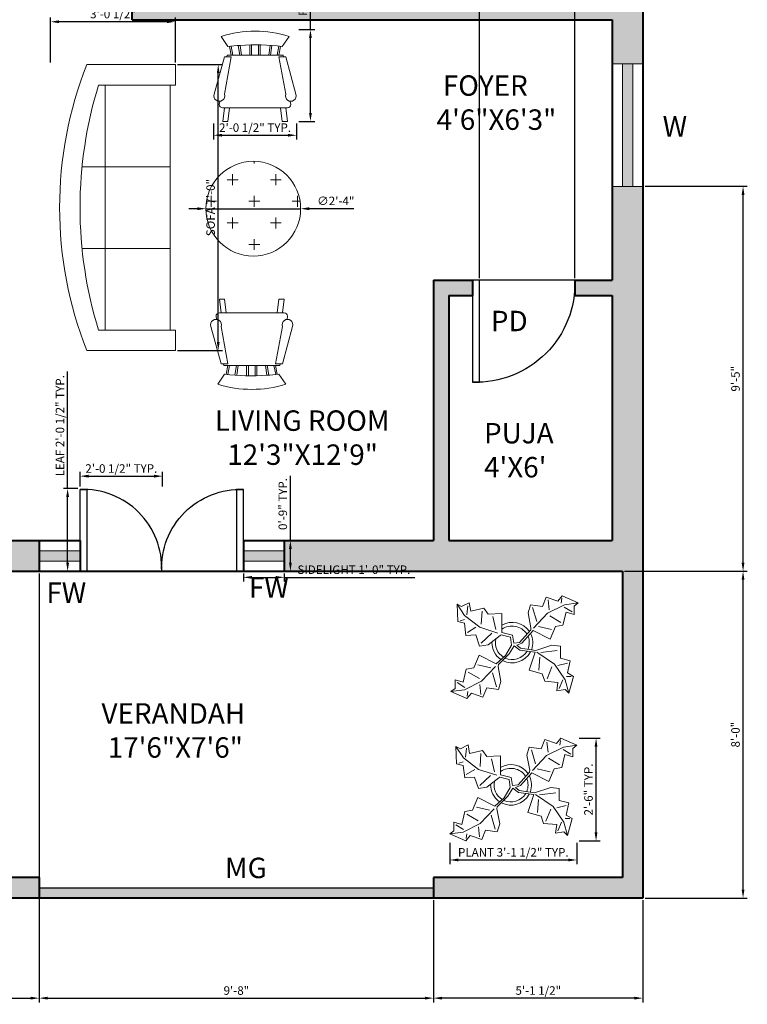
# Model space of a CAD drawing. Units: inches. Extents: x 4432 to 4859, y 8121 to 8698.
# Tile 2 of 4: x 4644 to 4858, y 8121 to 8410. Entities that reach past the tile are written whole.
import ezdxf

# ---------------------------------------------------------------- set-up
doc = ezdxf.new("R2010")
doc.units = ezdxf.units.IN
for name, color, linetype, lineweight in [('A-ANNO-DIMS', 2, 'Continuous', 18), ('A-ANNO-TEXT', 7, 'Continuous', 18), ('A-AREA-IDEN', 4, 'Continuous', 18), ('A-DOOR', 3, 'Continuous', 25), ('A-FURN', 8, 'Continuous', 18), ('A-FURN-PATT', 8, 'Continuous', 13), ('A-FURN-PLNT', 94, 'Continuous', 13), ('A-GLAZ', 4, 'Continuous', 20), ('A-GLAZ-PATT', 4, 'Continuous', 13), ('A-WALL', 7, 'Continuous', 40)]:
    doc.layers.add(name, color=color, linetype=linetype, lineweight=lineweight)
doc.layers.add('A-WALL-PATT', color=219, linetype='Continuous', lineweight=13, true_color=0x642165)
doc.styles.get("Standard").update_dxf_attribs({"font": 'arial.ttf'})
doc.dimstyles.new('ISO-25', dxfattribs={"dimtxt": 2.5, "dimasz": 2.5, "dimexe": 1.25, "dimexo": 0.625, "dimtad": 1, "dimlunit": 3, "dimtxsty": 'Standard', "dimcen": 2.5, "dimadec": 0, "dimazin": 0, "dimtfac": 1, "dimtmove": 0, "dimatfit": 3, "dimfxl": 1, "dimarcsym": 0})

# ---------------------------------------------------------------- blocks, each defined once
blk = doc.blocks.new('Chair - Rocking')
for p, q in [((-8, -4.5), (-10, -1.5)), ((8, -4.5), (10, -1.5)), ((-7.5, -4.5), (-7, -7)), ((-6.5, -7), (-7.02225, -4.43)), ((-4.5, -7), (-4.96674, -4.19951)), ((-4, -7), (-4.40532, -4.16272)), ((-1.5, -4.05012), (-1.5, -7)), ((-1, -7), (-1, -4.05012)), ((1, -7), (1, -4.04655)), ((1.5, -4.05012), (1.5, -7)), ((4, -7), (4.40187, -4.18694)), ((4.5, -7), (4.96761, -4.19437)), ((6.5, -7), (7, -4.4057)), ((7.5, -4.5), (7, -7)), ((-9, -7.5), (-12, -18.49999)), ((-7, -7.5), (-9, -7.5)), ((-9, -18.49999), (-7, -7.5)), ((-8.23428, -6.99939), (-8.3093, -7.47958)), ((-8.23041, -7), (8.23915, -7)), ((7, -7.5), (9, -7.5)), ((9, -18.49999), (7, -7.5)), ((8.31071, -7.48854), (8.23449, -7.00073)), ((9, -7.5), (12, -18.49999)), ((-10.36644, -20.64523), (-10.5, -21.49999)), ((-9, -22.49999), (-9.5, -26.49999)), ((0, -22.49999), (-9.5, -22.49999)), ((-8, -26.49999), (-7.5, -22.49999)), ((0, -22.49999), (9.5, -22.49999)), ((8, -26.49999), (7.5, -22.49999)), ((9, -22.49999), (9.5, -26.49999)), ((10.5, -21.49999), (10.3575, -20.58798)), ((-9.5, -26.49999), (-8, -26.49999)), ((9.5, -26.49999), (8, -26.49999))]:
    blk.add_line(p, q)
for centre, radius, start, end in [((0, -34.08333), 34.08333, 72.93847, 107.0615), ((0, -68.25004), 64.25, 93.92211, 97.15267), ((0, -68.25004), 64.25, 82.84733, 93.92211), ((-10.5, -18.99999), 1.58114, 161.5651, 18.43495), ((10.5, -18.99999), 1.58114, 161.5651, 18.43495), ((-9.5, -21.49999), 1, 180, 270), ((9.5, -21.49999), 1, 270, 0)]:
    blk.add_arc(centre, radius, start, end)
blk = doc.blocks.new('Plant - Rubber or Philodendron')
for p, q in [((-14.8639, 10.7964), (-12.6195, 11.8975)), ((-12.6195, 11.8975), (-12.1909, 9.4345)), ((8.8871, 10.7908), (9.9809, 13.4933)), ((9.9809, 13.4933), (13.3837, 12.301)), ((10.5828, 12.6946), (10.8893, 9.7953)), ((13.3837, 12.301), (14.68, 13.9039)), ((14.5816, 13.2037), (14.3848, 11.8033)), ((14.68, 13.9039), (19.3848, 11.8146)), ((19.3848, 11.8146), (15.3859, 11.3055)), ((19.3848, 11.8146), (18.1868, 10.9119)), ((-16.2005, 11.4774), (-13.9899, 8.1064)), ((-16.2005, 11.4774), (-14.8639, 10.7964)), ((-16.0159, 6.3329), (-16.2005, 11.4774)), ((-13.3174, 8.325), (-13.0735, 11.0065)), ((-12.1909, 9.4345), (-8.3829, 10.3)), ((-8.8369, 9.409), (-9.0894, 5.6095)), ((-8.3829, 10.3), (-7.0549, 8.501)), ((-7.0549, 8.501), (-3.0284, 8.6941)), ((-3.0284, 8.6941), (-3.0709, 3.1041)), ((4.6914, 8.8812), (5.3859, 11.2828)), ((4.6914, 8.8812), (5.5014, 4.4831)), ((5.3859, 11.2828), (8.8871, 10.7908)), ((5.9878, 10.4842), (7.1971, 6.3869)), ((10.3916, 8.7942), (6.2847, 4.4028)), ((15.3859, 11.3055), (10.3916, 8.7942)), ((15.7909, 9.1065), (14.8995, 5.3044)), ((15.2875, 10.6053), (17.5907, 9.2105)), ((18.1925, 8.4119), (15.7909, 9.1065)), ((18.1868, 10.9119), (18.1925, 8.4119)), ((-14.0069, 5.8704), (-16.0159, 6.3329)), ((-15.3434, 6.5514), (-13.9984, 6.9884)), ((-13.5868, 2.2894), (-14.0069, 5.8704)), ((-13.9899, 8.1064), (-9.5434, 4.7185)), ((-4.8529, 4.012), (-5.7184, 7.82)), ((14.2977, 6.1031), (10.9934, 7.9956)), ((-13.1329, 3.1804), (-10.6614, 4.727)), ((-9.5434, 4.7185), (-4.1917, 2.9888)), ((-9.1318, 0.0195), (-5.9793, 2.9025)), ((-3.0709, 3.1041), (0.0797, 2.3163)), ((2.1141, 0.2298), (5.4346, 3.9146)), ((6.1032, 3.6844), (2.8262, -0.031)), ((5.4346, 3.9146), (5.5014, 4.4831)), ((11.1089, 1.1958), (6.1032, 3.6844)), ((7.7005, 4.8881), (11.5025, 3.9967)), ((12.7005, 4.8994), (11.1089, 1.1958)), ((14.8995, 5.3044), (12.7005, 4.8994)), ((-10.6784, 2.491), (-13.5868, 2.2894)), ((-9.5858, -0.8715), (-10.6784, 2.491)), ((-7.1228, -0.443), (-3.5248, 2.2131)), ((-3.5248, 2.2131), (-3.3011, 2.4355)), ((-3.3011, 2.4355), (-0.5306, 1.7947)), ((-0.5306, 1.7947), (-0.2255, -0.5527)), ((-0.5306, 1.7947), (-0.5306, 1.7947)), ((0.0797, 2.3163), (0.4866, -0.031)), ((0.4866, -0.031), (2.1141, 0.2298)), ((-7.1228, -0.443), (-9.5858, -0.8715)), ((-2.019, -3.6148), (-0.2255, -0.5527)), ((-0.9375, -3.1608), (0.5883, -0.8135)), ((0.5883, -0.8135), (2.2447, -2.0916)), ((2.8262, -0.031), (1.3003, -0.5527)), ((1.3003, -0.5527), (2.4193, -1.4655)), ((2.2447, -2.0916), (6.7108, -2.6626)), ((2.4193, -1.4655), (6.895, -2.1175)), ((4.943, -7.9659), (6.7108, -2.6626)), ((11.6605, -0.5413), (6.895, -2.1175)), ((12.3677, -6.1981), (7.219, -2.6772)), ((8.3544, -2.7453), (13.1973, -2.1704)), ((11.6605, -0.5413), (14.1354, -0.8948)), ((14.1354, -0.8948), (14.1354, -4.4304)), ((-11.3237, -7.2629), (-9.7321, -3.5593)), ((-9.7321, -3.5593), (-4.7264, -6.0479)), ((-2.019, -3.6148), (-4.7264, -6.0479)), ((-4.0579, -6.2781), (-0.9375, -3.1608)), ((8.125, -4.0768), (7.7715, -7.9659)), ((14.1354, -4.4304), (16.9638, -5.1375)), ((16.9638, -5.1375), (16.2567, -8.673)), ((-14.4141, -11.4699), (-13.5228, -7.6679)), ((-13.5228, -7.6679), (-11.3237, -7.2629)), ((-12.921, -8.4665), (-9.6166, -10.359)), ((-6.3237, -7.2516), (-10.1257, -6.3602)), ((-9.0148, -11.1577), (-4.9047, -6.8122)), ((-4.1246, -6.8466), (-4.0579, -6.2781)), ((-3.3146, -11.2447), (-4.1246, -6.8466)), ((8.8321, -9.0266), (4.943, -7.9659)), ((10.2463, -10.4408), (11.6605, -6.9053)), ((15.5496, -10.7943), (12.3677, -6.1981)), ((16.2567, -5.8446), (13.4283, -6.5517)), ((16.2567, -8.673), (18.0245, -9.7337)), ((-16.8157, -10.7754), (-14.4141, -11.4699)), ((-16.8101, -13.2754), (-16.8157, -10.7754)), ((-14.0091, -13.669), (-9.0148, -11.1577)), ((-4.611, -12.8477), (-5.8203, -8.7504)), ((-3.3146, -11.2447), (-4.0092, -13.6463)), ((9.5392, -11.1479), (8.8321, -9.0266)), ((13.4283, -11.5015), (9.5392, -11.1479)), ((13.0748, -13.9763), (13.4283, -11.5015)), ((14.8425, -10.7943), (13.7819, -13.2692)), ((16.6103, -14.6834), (15.5496, -10.7943)), ((17.3174, -9.7337), (15.9032, -9.7337)), ((18.0245, -9.7337), (16.6103, -14.6834)), ((-18.008, -14.1781), (-16.8101, -13.2754)), ((-18.008, -14.1781), (-14.0091, -13.669)), ((-13.3032, -16.2674), (-18.008, -14.1781)), ((-13.9107, -12.9688), (-16.2139, -11.574)), ((-13.2048, -15.5672), (-13.008, -14.1668)), ((-9.206, -15.0581), (-9.5126, -12.1588)), ((-7.5103, -13.1543), (-8.6042, -15.8568)), ((-4.0092, -13.6463), (-7.5103, -13.1543)), ((15.5496, -13.6228), (13.0748, -13.9763)), ((16.6103, -14.6834), (15.5496, -13.6228)), ((-12.0069, -14.6645), (-13.3032, -16.2674)), ((-8.6042, -15.8568), (-12.0069, -14.6645))]:
    blk.add_line(p, q)
for centre, radius, start, end in [((0, 0), 6.1275, 34.37569, 120.1028), ((-0.0601, -0.2075), 5.2461, 33.82192, 124.9414), ((0.0308, 0.1664), 6, 178.6147, 235.1169), ((0.0308, 0.1664), 5, 168.1647, 238.6725), ((-0.2664, 0.1682), 5.2775, 338.4094, 20.03007), ((-0.098, 0.1364), 6.1288, 341.2017, 26.09184), ((-0.0234, 0.3825), 6.1492, 242.5812, 331.2714), ((-0.1102, 0.4886), 5.2883, 247.3711, 327.472)]:
    blk.add_arc(centre, radius, start, end)
blk = doc.blocks.new('Sofa - Roundback 7 ft.')
for p, q in [((-12.00002, -32.4421), (-12.00003, -6.5971)), ((11.99997, -32.4421), (11.99998, -6.5971)), ((-36.000027, -34), (-36.000027, -11.4696)), ((35.99998, -34), (35.99998, -11.4696)), ((-35.999844, -13.3819), (35.9998, -13.3819)), ((-36.000027, -32.4421), (35.99998, -32.4421))]:
    blk.add_line(p, q)
for points in [[(-36.000027, -34), (-42.000027, -34), (-42.000027, -8)], [(41.99998, -8), (41.99998, -34), (35.99998, -34)]]:
    blk.add_lwpolyline(points)
for centre, radius, start, end in [((0, -114.25), 114.25, 68.43141, 111.5686), ((-0.00001, -127.1968), 121.1968, 72.72033, 107.2797)]:
    blk.add_arc(centre, radius, start, end)
blk = doc.blocks.new('WIN-36IN')
for p, q in [((0, 0), (0, 9)), ((0, 9), (36, 9)), ((36, 9), (36, 0)), ((0, 6), (36, 6)), ((0, 3), (36, 3)), ((36, 0), (0, 0))]:
    blk.add_line(p, q)
blk = doc.blocks.new('SIDELIGHT-12IN')
for p, q in [((0, 9), (0, 0)), ((12, 9), (0, 9)), ((12, 0), (12, 9)), ((12, 6), (0, 6)), ((12, 3), (0, 3)), ((0, 0), (12, 0))]:
    blk.add_line(p, q)
blk = doc.blocks.new('DOOR-SWING-30IN')
for p, q in [((0, 30), (0, 0)), ((-30, 0), (-30, 2)), ((-30, 2), (0, 2)), ((0, 0), (-30, 0))]:
    blk.add_line(p, q)
blk.add_arc((-1, 1), 29.02, 88.0251, 181.9749)
blk = doc.blocks.new('ENTRY-LEAF-24IN')
for p, q in [((0, 0), (0, 24)), ((0, 24), (2, 24)), ((2, 24), (2, 0))]:
    blk.add_line(p, q)
blk.add_arc((1, 1), 23.02, 357.5104, 92.4896)
blk = doc.blocks.new('*D27')
at = {"layer": 'A-ANNO-DIMS', "color": 0, "lineweight": -2, "transparency": 16777216}
for p, q in [((4770.69, 8168.13), (4770.69, 8161.89)), ((4808.08, 8168.13), (4808.08, 8161.89)), ((4773.19, 8163.14), (4805.58, 8163.14))]:
    blk.add_line(p, q, dxfattribs=at)
at = {"layer": 'A-ANNO-DIMS', "color": 0, "transparency": 16777216}
for points in [[(4773.19, 8163.56), (4773.19, 8162.73), (4770.69, 8163.14)], [(4805.58, 8163.56), (4805.58, 8162.73), (4808.08, 8163.14)]]:
    blk.add_solid(points, dxfattribs=at)
at = {"layer": 'Defpoints', "color": 0, "transparency": 16777216}
for p in [(4770.69, 8168.75), (4808.08, 8168.75), (4808.08, 8163.14)]:
    blk.add_point(p, dxfattribs=at)
at = {"layer": 'A-ANNO-DIMS', "color": 0, "transparency": 16777216, "insert": (4789.38, 8165.06), "char_height": 2.5, "attachment_point": 5}
blk.add_mtext('PLANT 3\'-1 1/2" TYP.', dxfattribs=at)
blk = doc.blocks.new('*D28')
at = {"layer": 'A-ANNO-DIMS', "color": 0, "lineweight": -2, "transparency": 16777216}
for p, q in [((4808.7, 8198.92), (4814.94, 8198.92)), ((4813.69, 8171.25), (4813.69, 8196.42)), ((4808.7, 8168.75), (4814.94, 8168.75))]:
    blk.add_line(p, q, dxfattribs=at)
at = {"layer": 'A-ANNO-DIMS', "color": 0, "transparency": 16777216}
for points in [[(4813.27, 8196.42), (4814.1, 8196.42), (4813.69, 8198.92)], [(4813.27, 8171.25), (4814.1, 8171.25), (4813.69, 8168.75)]]:
    blk.add_solid(points, dxfattribs=at)
at = {"layer": 'Defpoints', "color": 0, "transparency": 16777216}
for p in [(4808.08, 8198.92), (4813.69, 8198.92), (4808.08, 8168.75)]:
    blk.add_point(p, dxfattribs=at)
at = {"layer": 'A-ANNO-DIMS', "color": 0, "transparency": 16777216, "insert": (4811.79, 8183.84), "char_height": 2.5, "attachment_point": 5, "rotation": 90}
blk.add_mtext('2\'-6" TYP.', dxfattribs=at)
blk = doc.blocks.new('*D33')
at = {"layer": 'A-ANNO-DIMS', "color": 0, "lineweight": -2, "transparency": 16777216}
for p, q in [((4729.79, 8407.06), (4729.79, 8441.83)), ((4726.37, 8407.06), (4731.04, 8407.06)), ((4729.79, 8382.56), (4729.79, 8404.56)), ((4726.37, 8380.06), (4731.04, 8380.06))]:
    blk.add_line(p, q, dxfattribs=at)
at = {"layer": 'A-ANNO-DIMS', "color": 0, "transparency": 16777216}
for points in [[(4729.38, 8404.56), (4730.21, 8404.56), (4729.79, 8407.06)], [(4729.38, 8382.56), (4730.21, 8382.56), (4729.79, 8380.06)]]:
    blk.add_solid(points, dxfattribs=at)
at = {"layer": 'Defpoints', "color": 0, "transparency": 16777216}
for p in [(4725.74, 8407.06), (4729.79, 8407.06), (4725.74, 8380.06)]:
    blk.add_point(p, dxfattribs=at)
at = {"layer": 'A-ANNO-DIMS', "color": 0, "transparency": 16777216, "insert": (4727.87, 8425.7), "char_height": 2.5, "attachment_point": 5, "rotation": 90}
blk.add_mtext('ROCKER 2\'-3" TYP.', dxfattribs=at)
blk = doc.blocks.new('*D34')
at = {"layer": 'A-ANNO-DIMS', "color": 0, "lineweight": -2, "transparency": 16777216}
for p, q in [((4701.31, 8379.44), (4701.31, 8374.76)), ((4725.74, 8379.44), (4725.74, 8374.76)), ((4703.81, 8376.01), (4723.24, 8376.01))]:
    blk.add_line(p, q, dxfattribs=at)
at = {"layer": 'A-ANNO-DIMS', "color": 0, "transparency": 16777216}
for points in [[(4703.81, 8376.43), (4703.81, 8375.6), (4701.31, 8376.01)], [(4723.24, 8376.43), (4723.24, 8375.6), (4725.74, 8376.01)]]:
    blk.add_solid(points, dxfattribs=at)
at = {"layer": 'Defpoints', "color": 0, "transparency": 16777216}
for p in [(4701.31, 8380.06), (4725.74, 8380.06), (4725.74, 8376.01)]:
    blk.add_point(p, dxfattribs=at)
at = {"layer": 'A-ANNO-DIMS', "color": 0, "transparency": 16777216, "insert": (4713.52, 8377.93), "char_height": 2.5, "attachment_point": 5}
blk.add_mtext('2\'-0 1/2" TYP.', dxfattribs=at)
blk = doc.blocks.new('*D39')
at = {"layer": 'A-ANNO-DIMS', "color": 0, "lineweight": -2, "transparency": 16777216}
for p, q in [((4710.1, 8247.33), (4710.1, 8244.91)), ((4712.6, 8246.16), (4719.6, 8246.16)), ((4722.1, 8247.33), (4722.1, 8244.91)), ((4722.1, 8246.16), (4760.49, 8246.16))]:
    blk.add_line(p, q, dxfattribs=at)
at = {"layer": 'A-ANNO-DIMS', "color": 0, "transparency": 16777216}
for points in [[(4712.6, 8246.57), (4712.6, 8245.74), (4710.1, 8246.16)], [(4719.6, 8246.57), (4719.6, 8245.74), (4722.1, 8246.16)]]:
    blk.add_solid(points, dxfattribs=at)
at = {"layer": 'Defpoints', "color": 0, "transparency": 16777216}
for p in [(4710.1, 8247.96), (4722.1, 8247.96), (4722.1, 8246.16)]:
    blk.add_point(p, dxfattribs=at)
at = {"layer": 'A-ANNO-DIMS', "color": 0, "transparency": 16777216, "insert": (4742.55, 8248.07), "char_height": 2.5, "attachment_point": 5}
blk.add_mtext('SIDELIGHT 1\'-0" TYP.', dxfattribs=at)
blk = doc.blocks.new('*D40')
at = {"layer": 'A-ANNO-DIMS', "color": 0, "lineweight": -2, "transparency": 16777216}
for p, q in [((4723.9, 8256.96), (4723.9, 8275.95)), ((4722.73, 8256.96), (4725.15, 8256.96)), ((4723.9, 8250.46), (4723.9, 8254.46)), ((4722.73, 8247.96), (4725.15, 8247.96))]:
    blk.add_line(p, q, dxfattribs=at)
at = {"layer": 'A-ANNO-DIMS', "color": 0, "transparency": 16777216}
for points in [[(4723.49, 8254.46), (4724.32, 8254.46), (4723.9, 8256.96)], [(4723.49, 8250.46), (4724.32, 8250.46), (4723.9, 8247.96)]]:
    blk.add_solid(points, dxfattribs=at)
at = {"layer": 'Defpoints', "color": 0, "transparency": 16777216}
for p in [(4722.1, 8256.96), (4723.9, 8256.96), (4722.1, 8247.96)]:
    blk.add_point(p, dxfattribs=at)
at = {"layer": 'A-ANNO-DIMS', "color": 0, "transparency": 16777216, "insert": (4722, 8267.7), "char_height": 2.5, "attachment_point": 5, "rotation": 90}
blk.add_mtext('0\'-9" TYP.', dxfattribs=at)
blk = doc.blocks.new('*D41')
at = {"layer": 'A-ANNO-DIMS', "color": 0, "lineweight": -2, "transparency": 16777216}
for p, q in [((4658.46, 8272.24), (4658.46, 8306.64)), ((4661.48, 8272.24), (4657.21, 8272.24)), ((4658.46, 8250.46), (4658.46, 8269.74)), ((4661.48, 8247.96), (4657.21, 8247.96))]:
    blk.add_line(p, q, dxfattribs=at)
at = {"layer": 'A-ANNO-DIMS', "color": 0, "transparency": 16777216}
for points in [[(4658.05, 8269.74), (4658.88, 8269.74), (4658.46, 8272.24)], [(4658.05, 8250.46), (4658.88, 8250.46), (4658.46, 8247.96)]]:
    blk.add_solid(points, dxfattribs=at)
at = {"layer": 'Defpoints', "color": 0, "transparency": 16777216}
for p in [(4658.46, 8272.24), (4662.1, 8272.24), (4662.1, 8247.96)]:
    blk.add_point(p, dxfattribs=at)
at = {"layer": 'A-ANNO-DIMS', "color": 0, "transparency": 16777216, "insert": (4656.54, 8290.69), "char_height": 2.5, "attachment_point": 5, "rotation": 90}
blk.add_mtext('LEAF 2\'-0 1/2" TYP.', dxfattribs=at)
blk = doc.blocks.new('*D42')
at = {"layer": 'A-ANNO-DIMS', "color": 0, "lineweight": -2, "transparency": 16777216}
for p, q in [((4662.1, 8272.86), (4662.1, 8277.13)), ((4664.6, 8275.88), (4683.88, 8275.88)), ((4686.38, 8272.86), (4686.38, 8277.13))]:
    blk.add_line(p, q, dxfattribs=at)
at = {"layer": 'A-ANNO-DIMS', "color": 0, "transparency": 16777216}
for points in [[(4664.6, 8276.3), (4664.6, 8275.46), (4662.1, 8275.88)], [(4683.88, 8276.3), (4683.88, 8275.46), (4686.38, 8275.88)]]:
    blk.add_solid(points, dxfattribs=at)
at = {"layer": 'Defpoints', "color": 0, "transparency": 16777216}
for p in [(4686.38, 8275.88), (4662.1, 8272.24), (4686.38, 8272.24)]:
    blk.add_point(p, dxfattribs=at)
at = {"layer": 'A-ANNO-DIMS', "color": 0, "transparency": 16777216, "insert": (4674.24, 8277.8), "char_height": 2.5, "attachment_point": 5}
blk.add_mtext('2\'-0 1/2" TYP.', dxfattribs=at)
blk = doc.blocks.new('*D49')
at = {"layer": 'A-ANNO-DIMS', "color": 0, "lineweight": -2, "transparency": 16777216}
for p, q in [((4690.73, 8396.76), (4703.96, 8396.76)), ((4702.71, 8315.26), (4702.71, 8394.26)), ((4690.73, 8312.76), (4703.96, 8312.76))]:
    blk.add_line(p, q, dxfattribs=at)
at = {"layer": 'A-ANNO-DIMS', "color": 0, "transparency": 16777216}
for points in [[(4702.29, 8394.26), (4703.12, 8394.26), (4702.71, 8396.76)], [(4702.29, 8315.26), (4703.12, 8315.26), (4702.71, 8312.76)]]:
    blk.add_solid(points, dxfattribs=at)
at = {"layer": 'Defpoints', "color": 0, "transparency": 16777216}
for p in [(4690.11, 8396.76), (4702.71, 8396.76), (4690.11, 8312.76)]:
    blk.add_point(p, dxfattribs=at)
at = {"layer": 'A-ANNO-DIMS', "color": 0, "transparency": 16777216, "insert": (4700.79, 8354.76), "char_height": 2.5, "attachment_point": 5, "rotation": 90}
blk.add_mtext('SOFA 7\'-0"', dxfattribs=at)
blk = doc.blocks.new('*D50')
at = {"layer": 'A-ANNO-DIMS', "color": 0, "lineweight": -2, "transparency": 16777216}
for p, q in [((4653.44, 8397.38), (4653.44, 8410.61)), ((4690.11, 8397.38), (4690.11, 8410.61)), ((4687.61, 8409.36), (4655.94, 8409.36))]:
    blk.add_line(p, q, dxfattribs=at)
at = {"layer": 'A-ANNO-DIMS', "color": 0, "transparency": 16777216}
for points in [[(4655.94, 8409.77), (4655.94, 8408.94), (4653.44, 8409.36)], [(4687.61, 8409.77), (4687.61, 8408.94), (4690.11, 8409.36)]]:
    blk.add_solid(points, dxfattribs=at)
at = {"layer": 'Defpoints', "color": 0, "transparency": 16777216}
for p in [(4653.44, 8409.36), (4653.44, 8396.76), (4690.11, 8396.76)]:
    blk.add_point(p, dxfattribs=at)
at = {"layer": 'A-ANNO-DIMS', "color": 0, "transparency": 16777216, "insert": (4671.77, 8411.28), "char_height": 2.5, "attachment_point": 5}
blk.add_mtext('3\'-0 1/2"', dxfattribs=at)
blk = doc.blocks.new('*D55')
at = {"layer": 'A-ANNO-DIMS', "color": 0, "lineweight": -2, "transparency": 16777216}
for p, q in [((4822.09, 8247.96), (4858.12, 8247.96)), ((4856.87, 8154.46), (4856.87, 8245.46)), ((4828.09, 8151.96), (4858.12, 8151.96))]:
    blk.add_line(p, q, dxfattribs=at)
at = {"layer": 'A-ANNO-DIMS', "color": 0, "transparency": 16777216}
for points in [[(4856.45, 8245.46), (4857.28, 8245.46), (4856.87, 8247.96)], [(4856.45, 8154.46), (4857.28, 8154.46), (4856.87, 8151.96)]]:
    blk.add_solid(points, dxfattribs=at)
at = {"layer": 'Defpoints', "color": 0, "transparency": 16777216}
for p in [(4821.47, 8247.96), (4856.87, 8247.96), (4827.47, 8151.96)]:
    blk.add_point(p, dxfattribs=at)
at = {"layer": 'A-ANNO-DIMS', "color": 0, "transparency": 16777216, "insert": (4854.97, 8199.96), "char_height": 2.5, "attachment_point": 5, "rotation": 90}
blk.add_mtext('8\'-0"', dxfattribs=at)
blk = doc.blocks.new('*D56')
at = {"layer": 'A-ANNO-DIMS', "color": 0, "lineweight": -2, "transparency": 16777216}
for p, q in [((4765.97, 8151.33), (4765.97, 8121.31)), ((4827.47, 8151.33), (4827.47, 8121.31)), ((4824.97, 8122.56), (4768.47, 8122.56))]:
    blk.add_line(p, q, dxfattribs=at)
at = {"layer": 'A-ANNO-DIMS', "color": 0, "transparency": 16777216}
for points in [[(4768.47, 8122.97), (4768.47, 8122.14), (4765.97, 8122.56)], [(4824.97, 8122.97), (4824.97, 8122.14), (4827.47, 8122.56)]]:
    blk.add_solid(points, dxfattribs=at)
at = {"layer": 'Defpoints', "color": 0, "transparency": 16777216}
for p in [(4765.97, 8151.96), (4827.47, 8151.96), (4765.97, 8122.56)]:
    blk.add_point(p, dxfattribs=at)
at = {"layer": 'A-ANNO-DIMS', "color": 0, "transparency": 16777216, "insert": (4796.72, 8124.47), "char_height": 2.5, "attachment_point": 5}
blk.add_mtext('5\'-1 1/2"', dxfattribs=at)
blk = doc.blocks.new('*D57')
at = {"layer": 'A-ANNO-DIMS', "color": 0, "lineweight": -2, "transparency": 16777216}
for p, q in [((4650.1, 8151.33), (4650.1, 8121.31)), ((4765.97, 8151.33), (4765.97, 8121.31)), ((4652.6, 8122.56), (4763.47, 8122.56))]:
    blk.add_line(p, q, dxfattribs=at)
at = {"layer": 'A-ANNO-DIMS', "color": 0, "transparency": 16777216}
for points in [[(4652.6, 8122.97), (4652.6, 8122.14), (4650.1, 8122.56)], [(4763.47, 8122.97), (4763.47, 8122.14), (4765.97, 8122.56)]]:
    blk.add_solid(points, dxfattribs=at)
at = {"layer": 'Defpoints', "color": 0, "transparency": 16777216}
for p in [(4650.1, 8151.96), (4765.97, 8151.96), (4765.97, 8122.56)]:
    blk.add_point(p, dxfattribs=at)
at = {"layer": 'A-ANNO-DIMS', "color": 0, "transparency": 16777216, "insert": (4708.04, 8124.46), "char_height": 2.5, "attachment_point": 5}
blk.add_mtext('9\'-8"', dxfattribs=at)
blk = doc.blocks.new('*D62')
at = {"layer": 'A-ANNO-DIMS', "color": 0, "lineweight": -2, "transparency": 16777216}
for p, q in [((4617.47, 8256.33), (4617.47, 8121.31)), ((4650.1, 8247.33), (4650.1, 8121.31)), ((4619.97, 8122.56), (4647.6, 8122.56))]:
    blk.add_line(p, q, dxfattribs=at)
at = {"layer": 'A-ANNO-DIMS', "color": 0, "transparency": 16777216}
for points in [[(4619.97, 8122.97), (4619.97, 8122.14), (4617.47, 8122.56)], [(4647.6, 8122.97), (4647.6, 8122.14), (4650.1, 8122.56)]]:
    blk.add_solid(points, dxfattribs=at)
at = {"layer": 'Defpoints', "color": 0, "transparency": 16777216}
for p in [(4617.47, 8256.96), (4650.1, 8247.96), (4650.1, 8122.56)]:
    blk.add_point(p, dxfattribs=at)
at = {"layer": 'A-ANNO-DIMS', "color": 0, "transparency": 16777216, "insert": (4633.79, 8124.47), "char_height": 2.5, "attachment_point": 5}
blk.add_mtext('2\'-8 1/2"', dxfattribs=at)
blk = doc.blocks.new('*D65')
at = {"layer": 'A-ANNO-DIMS', "color": 0, "lineweight": -2, "transparency": 16777216}
for p, q in [((4828.09, 8361.01), (4858.12, 8361.01)), ((4856.87, 8250.46), (4856.87, 8358.51)), ((4822.09, 8247.96), (4858.12, 8247.96))]:
    blk.add_line(p, q, dxfattribs=at)
at = {"layer": 'A-ANNO-DIMS', "color": 0, "transparency": 16777216}
for points in [[(4856.45, 8358.51), (4857.28, 8358.51), (4856.87, 8361.01)], [(4856.45, 8250.46), (4857.28, 8250.46), (4856.87, 8247.96)]]:
    blk.add_solid(points, dxfattribs=at)
at = {"layer": 'Defpoints', "color": 0, "transparency": 16777216}
for p in [(4827.47, 8361.01), (4856.87, 8361.01), (4821.47, 8247.96)]:
    blk.add_point(p, dxfattribs=at)
at = {"layer": 'A-ANNO-DIMS', "color": 0, "transparency": 16777216, "insert": (4854.97, 8304.48), "char_height": 2.5, "attachment_point": 5, "rotation": 90}
blk.add_mtext('9\'-5"', dxfattribs=at)
blk = doc.blocks.new('*D69')
at = {"layer": 'A-ANNO-DIMS', "color": 0, "lineweight": -2, "transparency": 16777216}
for p, q in [((4779.44, 8334.08), (4779.44, 8662.61)), ((4807.44, 8334.08), (4807.44, 8662.61)), ((4781.94, 8661.36), (4804.94, 8661.36))]:
    blk.add_line(p, q, dxfattribs=at)
at = {"layer": 'A-ANNO-DIMS', "color": 0, "transparency": 16777216}
for points in [[(4781.94, 8661.77), (4781.94, 8660.94), (4779.44, 8661.36)], [(4804.94, 8661.77), (4804.94, 8660.94), (4807.44, 8661.36)]]:
    blk.add_solid(points, dxfattribs=at)
at = {"layer": 'Defpoints', "color": 0, "transparency": 16777216}
for p in [(4807.44, 8661.36), (4779.44, 8333.46), (4807.44, 8333.46)]:
    blk.add_point(p, dxfattribs=at)
at = {"layer": 'A-ANNO-DIMS', "color": 0, "transparency": 16777216, "insert": (4793.44, 8663.24), "char_height": 2.5, "attachment_point": 5}
blk.add_mtext('2\'-4"', dxfattribs=at)
blk = doc.blocks.new('*D74')
at = {"layer": 'A-ANNO-DIMS', "color": 0, "lineweight": -2, "transparency": 16777216}
for p, q in [((4696.59, 8354.44), (4694.09, 8354.44)), ((4699.09, 8354.44), (4726.92, 8354.44)), ((4742.53, 8354.44), (4729.42, 8354.44))]:
    blk.add_line(p, q, dxfattribs=at)
at = {"layer": 'A-ANNO-DIMS', "color": 0, "transparency": 16777216}
for points in [[(4696.59, 8354.86), (4696.59, 8354.02), (4699.09, 8354.44)], [(4729.42, 8354.86), (4729.42, 8354.02), (4726.92, 8354.44)]]:
    blk.add_solid(points, dxfattribs=at)
at = {"layer": 'Defpoints', "color": 0, "transparency": 16777216}
for p in [(4699.09, 8354.44), (4726.92, 8354.44)]:
    blk.add_point(p, dxfattribs=at)
at = {"layer": 'A-ANNO-DIMS', "color": 0, "transparency": 16777216, "insert": (4737.23, 8356.41), "char_height": 2.5, "attachment_point": 5, "rotation": 359.999}
blk.add_mtext('∅2\'-4"', dxfattribs=at)

msp = doc.modelspace()

# ---------------------------------------------------------------- hatches: boundary and pattern name
at = {"layer": 'A-FURN-PATT'}
h = msp.add_hatch(dxfattribs=at)
h.set_pattern_fill('CROSS', color=256)
h.paths.add_polyline_path([(4558.735, 8563.044), (4508.335, 8563.044), (4508.335, 8547.844), (4495.535, 8547.844), (4495.535, 8503.044), (4558.735, 8503.044)])
h.paths.add_polyline_path([(4768.654, 8563.044), (4718.254, 8563.044), (4718.254, 8547.844), (4705.454, 8547.844), (4705.454, 8503.044), (4768.654, 8503.044)])
h.paths.add_polyline_path([(4699.088, 8354.439, 1), (4726.919, 8354.439, 1)])
at = {"layer": 'A-GLAZ-PATT'}
h = msp.add_hatch(color=256, dxfattribs=at)
h.dxf.hatch_style = 1
h.paths.add_polyline_path([(4592.313, 8628.956), (4556.313, 8628.956), (4556.313, 8625.956), (4592.313, 8625.956)])
h.paths.add_polyline_path([(4660.176, 8628.956), (4636.176, 8628.956), (4636.176, 8625.956), (4660.176, 8625.956)])
h.paths.add_polyline_path([(4799.877, 8628.956), (4763.877, 8628.956), (4763.877, 8625.956), (4799.877, 8625.956)])
h.paths.add_polyline_path([(4473.468, 8508.361), (4470.468, 8508.361), (4470.468, 8448.361), (4473.468, 8448.361)])
h.paths.add_polyline_path([(4473.468, 8398.047), (4470.468, 8398.047), (4470.468, 8377.047), (4473.468, 8377.047)])
h.paths.add_polyline_path([(4473.468, 8341.903), (4470.468, 8341.903), (4470.468, 8305.903), (4473.468, 8305.903)])
h.paths.add_polyline_path([(4577.354, 8253.956), (4529.354, 8253.956), (4529.354, 8250.956), (4577.354, 8250.956)])
h.paths.add_polyline_path([(4662.104, 8253.956), (4650.104, 8253.956), (4650.104, 8250.956), (4662.104, 8250.956)])
h.paths.add_polyline_path([(4722.104, 8253.956), (4710.104, 8253.956), (4710.104, 8250.956), (4722.104, 8250.956)])
h.paths.add_polyline_path([(4824.468, 8397.007), (4821.468, 8397.007), (4821.468, 8361.007), (4824.468, 8361.007)])
h.paths.add_polyline_path([(4824.468, 8509.871), (4821.468, 8509.871), (4821.468, 8449.871), (4824.468, 8449.871)])
at = {"layer": 'A-WALL-PATT'}
h = msp.add_hatch(color=256, dxfattribs=at)
h.dxf.hatch_style = 1
h.paths.add_polyline_path([(4556.313, 8631.956), (4467.468, 8631.956), (4467.468, 8508.361), (4476.468, 8508.361), (4476.468, 8622.956), (4556.313, 8622.956)])
h.paths.add_polyline_path([(4636.176, 8631.956), (4592.313, 8631.956), (4592.313, 8622.956), (4608.468, 8622.956), (4608.468, 8546.941), (4617.468, 8546.941), (4617.468, 8622.956), (4636.176, 8622.956)])
h.paths.add_polyline_path([(4763.877, 8631.956), (4660.176, 8631.956), (4660.176, 8622.956), (4677.468, 8622.956), (4677.468, 8502.956), (4617.468, 8502.956), (4617.468, 8524.355), (4608.468, 8524.355), (4608.468, 8459.776), (4615.468, 8459.776, -0.0172363), (4617.468, 8459.776), (4617.468, 8493.956), (4677.468, 8493.956), (4677.468, 8459.776, -0.0172363), (4679.468, 8459.776), (4686.468, 8459.776), (4686.468, 8622.956), (4763.877, 8622.956)])
h.paths.add_polyline_path([(4827.468, 8631.956), (4799.877, 8631.956), (4799.877, 8622.956), (4818.468, 8622.956), (4818.468, 8509.871), (4827.468, 8509.871)])
h.paths.add_polyline_path([(4617.468, 8429.776), (4608.468, 8429.776), (4608.468, 8418.956), (4476.468, 8418.956), (4476.468, 8448.361), (4467.468, 8448.361), (4467.468, 8398.047), (4476.468, 8398.047), (4476.468, 8409.956), (4608.468, 8409.956), (4608.468, 8397.41), (4612.05, 8397.41, -0.0497121), (4617.468, 8397.41)])
h.paths.add_polyline_path([(4827.468, 8449.871), (4818.468, 8449.871), (4818.468, 8418.956), (4686.468, 8418.956), (4686.468, 8429.776), (4677.468, 8429.776), (4677.468, 8409.956), (4818.468, 8409.956), (4818.468, 8397.007), (4827.468, 8397.007)])
h.paths.add_polyline_path([(4617.468, 8369.235), (4608.468, 8369.235), (4608.468, 8361.956), (4476.468, 8361.956), (4476.468, 8377.047), (4467.468, 8377.047), (4467.468, 8341.903), (4476.468, 8341.903), (4476.468, 8352.956), (4617.468, 8352.956)])
h.paths.add_polyline_path([(4529.354, 8256.956), (4476.468, 8256.956), (4476.468, 8305.903), (4467.468, 8305.903), (4467.468, 8151.956), (4650.104, 8151.956), (4650.104, 8157.956), (4471.968, 8157.956), (4471.968, 8169.956), (4599.396, 8169.956), (4599.396, 8174.456), (4476.468, 8174.456), (4476.468, 8247.956), (4529.354, 8247.956)])
h.paths.add_polyline_path([(4650.104, 8256.956), (4617.468, 8256.956), (4617.468, 8304.956), (4608.468, 8304.956), (4608.468, 8256.956), (4577.354, 8256.956), (4577.354, 8247.956), (4650.104, 8247.956)], flags=17)
h.paths.add_polyline_path([(4827.468, 8361.007), (4818.468, 8361.007), (4818.468, 8333.456), (4807.435, 8333.456, -0.0172363), (4807.435, 8331.456), (4807.435, 8328.956), (4818.468, 8328.956), (4818.468, 8256.956), (4770.468, 8256.956), (4770.468, 8328.956), (4777.435, 8328.956), (4777.435, 8333.456), (4765.968, 8333.456), (4765.968, 8256.956), (4722.104, 8256.956), (4722.104, 8247.956), (4821.468, 8247.956), (4821.468, 8157.956), (4765.968, 8157.956), (4765.968, 8151.956), (4827.468, 8151.956)])
h.paths.add_polyline_path([(4765.968, 8154.956), (4650.104, 8154.956), (4650.104, 8151.956), (4765.968, 8151.956)])

# ---------------------------------------------------------------- linework, layer by layer
at = {"layer": 'A-DOOR'}
for p, q in [((4807.435, 8333.456), (4777.435, 8333.456)), ((4662.104, 8247.956), (4710.104, 8247.956)), ((4710.104, 8247.956), (4686.104, 8247.956)), ((4650.104, 8154.956), (4765.968, 8154.956))]:
    msp.add_line(p, q, dxfattribs=at)
at = {"layer": 'A-FURN'}
msp.add_circle((4713.004, 8354.439), 13.915, dxfattribs=at)
at = {"layer": 'A-WALL'}
for p, q in [((4827.468, 8631.956), (4827.468, 8151.956)), ((4677.468, 8409.956), (4677.468, 8429.776)), ((4677.468, 8409.956), (4818.468, 8409.956)), ((4818.468, 8409.956), (4818.468, 8333.456)), ((4765.968, 8333.456), (4765.968, 8256.956)), ((4765.968, 8333.456), (4777.435, 8333.456)), ((4777.435, 8333.456), (4777.435, 8328.956)), ((4807.435, 8333.456), (4807.435, 8328.956)), ((4807.435, 8333.456), (4818.468, 8333.456)), ((4770.468, 8328.956), (4770.468, 8256.956)), ((4770.468, 8328.956), (4777.435, 8328.956)), ((4807.435, 8328.956), (4818.468, 8328.956)), ((4818.468, 8328.956), (4818.468, 8256.956)), ((4617.468, 8256.956), (4662.104, 8256.956)), ((4650.104, 8256.956), (4650.104, 8247.956)), ((4662.104, 8256.956), (4662.104, 8247.956)), ((4710.104, 8256.956), (4710.104, 8247.956)), ((4710.104, 8256.956), (4765.968, 8256.956)), ((4722.104, 8256.956), (4722.104, 8247.956)), ((4770.468, 8256.956), (4818.468, 8256.956)), ((4476.468, 8247.956), (4821.468, 8247.956)), ((4821.468, 8247.956), (4821.468, 8157.956)), ((4650.104, 8157.956), (4471.968, 8157.956)), ((4650.104, 8157.956), (4650.104, 8151.956)), ((4821.468, 8157.956), (4765.968, 8157.956)), ((4765.968, 8157.956), (4765.968, 8151.956)), ((4827.468, 8151.956), (4467.468, 8151.956))]:
    msp.add_line(p, q, dxfattribs=at)

# ---------------------------------------------------------------- block references
at = {"layer": 'A-DOOR', "extrusion": (0, 0, -1), "zscale": -1, "rotation": 90.00000000000492}
msp.add_blockref('DOOR-SWING-30IN', (-4777.435, 8333.456), dxfattribs=at)
at = {"layer": 'A-DOOR'}
msp.add_blockref('ENTRY-LEAF-24IN', (4662.104, 8247.956), dxfattribs=at)
at = {"layer": 'A-DOOR', "extrusion": (0, 0, -1), "zscale": -1}
msp.add_blockref('ENTRY-LEAF-24IN', (-4710.104, 8247.956), dxfattribs=at)
at = {"layer": 'A-FURN'}
msp.add_blockref('Chair - Rocking', (4713.525, 8406.562), dxfattribs=at)
for name, p, rotation in [('Sofa - Roundback 7 ft.', (4656.107, 8354.758), 89.99999999999999), ('Chair - Rocking', (4712.554, 8301.359), 180)]:
    msp.add_blockref(name, p, dxfattribs=dict(at, rotation=rotation))
at = {"layer": 'A-FURN-PLNT'}
for p in [(4789.071, 8226.815), (4788.695, 8185.018)]:
    msp.add_blockref('Plant - Rubber or Philodendron', p, dxfattribs=at)
at = {"layer": 'A-GLAZ', "rotation": 89.99999999999046}
msp.add_blockref('WIN-36IN', (4827.468, 8361.007), dxfattribs=at)
at = {"layer": 'A-GLAZ'}
for p in [(4650.104, 8247.956), (4710.104, 8247.956)]:
    msp.add_blockref('SIDELIGHT-12IN', p, dxfattribs=at)

# ---------------------------------------------------------------- texts
at = {"layer": 'A-ANNO-TEXT', "char_height": 6, "attachment_point": 1}
for s, insert in [('W  ', (4833.252, 8381.624)), ('PD', (4782.787, 8324.456)), ('FW', (4711.729, 8246.165)), ('FW', (4652.223, 8244.664)), ('MG', (4704.697, 8163.81))]:
    msp.add_mtext_dynamic_manual_height_columns(s, width=117.51606, gutter_width=12.5, heights=[0], dxfattribs=dict(at, insert=insert))
at = {"layer": 'A-AREA-IDEN', "char_height": 6, "attachment_point": 1}
for s, insert in [(' FOYER\\P4\'6"X6\'3"', (4766.845, 8393.604)), (' { LIVING ROOM\\P    12\'3"X12\'9"}', (4698.029, 8295.194)), (" PUJA\\P 4'X6'", (4778.952, 8291.499)), (' VERANDAH\\P  17\'6"X7\'6"', (4666.575, 8209.185))]:
    msp.add_mtext_dynamic_manual_height_columns(s, width=117.51606, gutter_width=12.5, heights=[0], dxfattribs=dict(at, insert=insert))

# ---------------------------------------------------------------- dimensions: what is measured, and where the dimension line sits
at = {"layer": 'A-ANNO-DIMS'}
for base, p1, p2, picture, middle in [((4807.435, 8661.356), (4779.435, 8333.456), (4807.435, 8333.456), '*D69', (4793.435, 8663.237)), ((4650.104, 8122.556), (4617.468, 8256.956), (4650.104, 8247.956), '*D62', (4633.786, 8124.474)), ((4765.968, 8122.556), (4650.104, 8151.956), (4765.968, 8151.956), '*D57', (4708.036, 8124.458)), ((4765.968, 8122.556), (4827.468, 8151.956), (4765.968, 8151.956), '*D56', (4796.718, 8124.474))]:
    dim = msp.add_linear_dim(base=base, p1=p1, p2=p2, dimstyle='ISO-25', override={"dimdec": 1, "dimlfac": 1, "dimrnd": 0, "dimzin": 1, "dimdsep": 46, "dimlunit": 4, "dimfrac": 2}, dxfattribs=at)
    dim.commit()
    dim.dimension.update_dxf_attribs({"geometry": picture, "text_midpoint": middle})
for base, p1, p2, text, picture, middle in [((4729.792, 8407.062), (4725.742, 8380.062), (4725.742, 8407.062), 'ROCKER <> TYP.', '*D33', (4727.873, 8425.698)), ((4702.707, 8396.758), (4690.107, 8312.758), (4690.107, 8396.758), 'SOFA <>', '*D49', (4700.788, 8354.758)), ((4658.462, 8272.237), (4662.104, 8247.956), (4662.104, 8272.237), 'LEAF <> TYP.', '*D41', (4656.544, 8290.691)), ((4723.904, 8256.956), (4722.104, 8247.956), (4722.104, 8256.956), '<> TYP.', '*D40', (4722.003, 8267.701)), ((4813.688, 8198.922), (4808.079, 8168.751), (4808.079, 8198.922), '<> TYP.', '*D28', (4811.787, 8183.837))]:
    dim = msp.add_linear_dim(base=base, p1=p1, p2=p2, angle=90, text=text, dimstyle='ISO-25', override={"dimdec": 1, "dimlfac": 1, "dimrnd": 0, "dimzin": 1, "dimdsep": 46, "dimlunit": 4, "dimfrac": 2}, dxfattribs=at)
    dim.commit()
    dim.dimension.update_dxf_attribs({"geometry": picture, "text_midpoint": middle})
for base, p1, p2, angle, picture, middle in [((4653.44, 8409.358), (4690.107, 8396.758), (4653.44, 8396.758), 180, '*D50', (4671.773, 8411.277)), ((4856.868, 8361.007), (4821.468, 8247.956), (4827.468, 8361.007), 90, '*D65', (4854.966, 8304.482)), ((4856.868, 8247.956), (4827.468, 8151.956), (4821.468, 8247.956), 90, '*D55', (4854.966, 8199.956))]:
    dim = msp.add_linear_dim(base=base, p1=p1, p2=p2, angle=angle, dimstyle='ISO-25', override={"dimdec": 1, "dimlfac": 1, "dimrnd": 0, "dimzin": 1, "dimdsep": 46, "dimlunit": 4, "dimfrac": 2}, dxfattribs=at)
    dim.commit()
    dim.dimension.update_dxf_attribs({"geometry": picture, "text_midpoint": middle})
for base, p1, p2, text, picture, middle in [((4725.742, 8376.012), (4701.307, 8380.062), (4725.742, 8380.062), '<> TYP.', '*D34', (4713.525, 8377.93)), ((4686.384, 8275.879), (4662.104, 8272.237), (4686.384, 8272.237), '<> TYP.', '*D42', (4674.244, 8277.796)), ((4722.104, 8246.156), (4710.104, 8247.956), (4722.104, 8247.956), 'SIDELIGHT <> TYP.', '*D39', (4742.546, 8248.074)), ((4808.079, 8163.142), (4770.687, 8168.751), (4808.079, 8168.751), 'PLANT <> TYP.', '*D27', (4789.383, 8165.061))]:
    dim = msp.add_linear_dim(base=base, p1=p1, p2=p2, text=text, dimstyle='ISO-25', override={"dimdec": 1, "dimlfac": 1, "dimrnd": 0, "dimzin": 1, "dimdsep": 46, "dimlunit": 4, "dimfrac": 2}, dxfattribs=at)
    dim.commit()
    dim.dimension.update_dxf_attribs({"geometry": picture, "text_midpoint": middle})
dim = msp.add_diameter_dim_2p(p1=(4699.088, 8354.439), p2=(4726.919, 8354.439), dimstyle='ISO-25', override={"dimdec": 1, "dimlfac": 1, "dimrnd": 0, "dimzin": 1, "dimdsep": 46, "dimlunit": 4, "dimfrac": 2}, dxfattribs=at)
dim.commit()
dim.dimension.update_dxf_attribs({"geometry": '*D74', "text_midpoint": (4737.227, 8354.439), "dimtype": 163})

doc.saveas('drawing.dxf')
